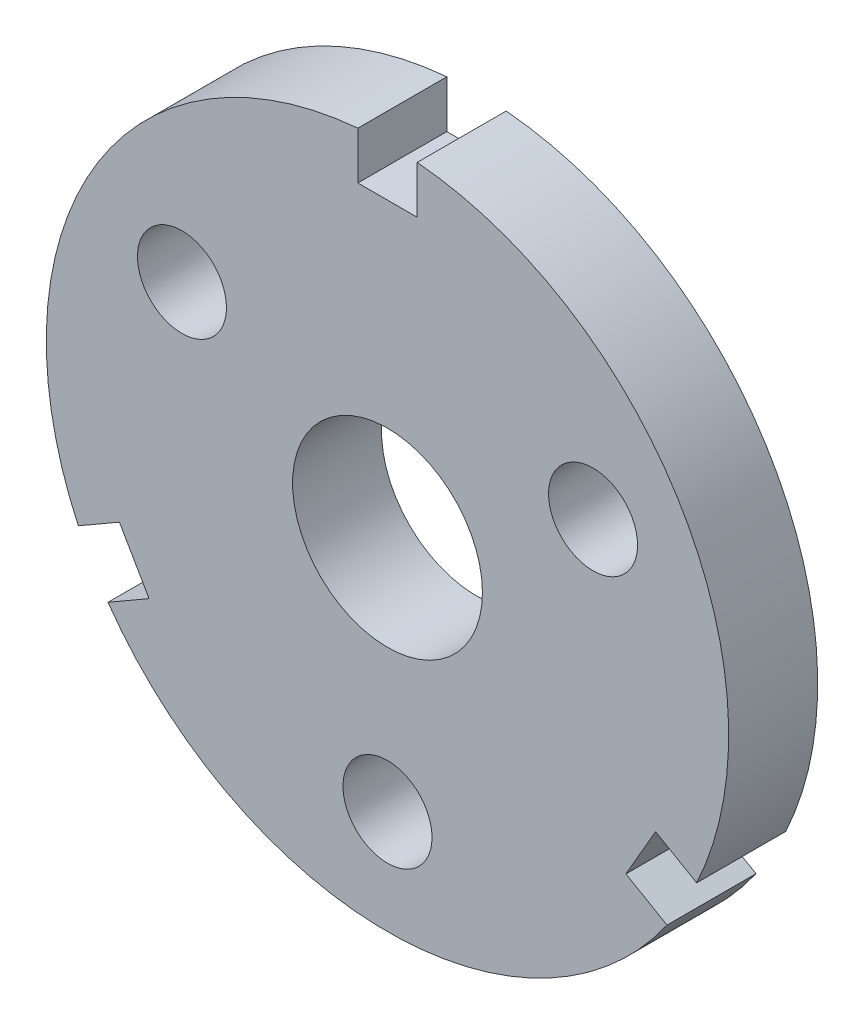
ISO-10303-21;
HEADER;
FILE_DESCRIPTION(('STEP AP214'),'2;1');
FILE_NAME('part.step','',(''),(''),'','','');
FILE_SCHEMA(('AUTOMOTIVE_DESIGN { 1 0 10303 214 1 1 1 1 }'));
ENDSEC;
DATA;
#1=APPLICATION_CONTEXT('core data for automotive mechanical design processes');
#2=APPLICATION_PROTOCOL_DEFINITION('international standard','automotive_design',2000,#1);
#3=PRODUCT_CONTEXT('',#1,'mechanical');
#4=PRODUCT('Part','Part','',(#3));
#5=PRODUCT_RELATED_PRODUCT_CATEGORY('part','',(#4));
#6=PRODUCT_DEFINITION_FORMATION('','',#4);
#7=PRODUCT_DEFINITION_CONTEXT('part definition',#1,'design');
#8=PRODUCT_DEFINITION('design','',#6,#7);
#9=PRODUCT_DEFINITION_SHAPE('','',#8);
#10=(LENGTH_UNIT() NAMED_UNIT(*) SI_UNIT(.MILLI.,.METRE.));
#11=(NAMED_UNIT(*) PLANE_ANGLE_UNIT() SI_UNIT($,.RADIAN.));
#12=(NAMED_UNIT(*) SI_UNIT($,.STERADIAN.) SOLID_ANGLE_UNIT());
#13=UNCERTAINTY_MEASURE_WITH_UNIT(LENGTH_MEASURE(1.E-05),#10,'distance_accuracy_value','');
#14=(GEOMETRIC_REPRESENTATION_CONTEXT(3) GLOBAL_UNCERTAINTY_ASSIGNED_CONTEXT((#13)) GLOBAL_UNIT_ASSIGNED_CONTEXT((#10,
#11,#12)) REPRESENTATION_CONTEXT('',''));
#15=CARTESIAN_POINT('',(0.,0.,0.));
#16=DIRECTION('',(0.,0.,1.));
#17=DIRECTION('',(1.,0.,0.));
#18=AXIS2_PLACEMENT_3D('',#15,#16,#17);
#19=CARTESIAN_POINT('',(0.,0.,15.));
#20=DIRECTION('',(0.,0.,-1.));
#21=DIRECTION('',(-1.,0.,0.));
#22=AXIS2_PLACEMENT_3D('',#19,#20,#21);
#23=CYLINDRICAL_SURFACE('',#22,57.5);
#24=CARTESIAN_POINT('',(0.,0.,0.));
#25=DIRECTION('',(0.,0.,1.));
#26=DIRECTION('',(1.,0.,0.));
#27=AXIS2_PLACEMENT_3D('',#24,#25,#26);
#28=CIRCLE('',#27,57.5);
#29=CARTESIAN_POINT('',(52.1078370824597,-24.3109710745512,0.));
#30=VERTEX_POINT('',#29);
#31=CARTESIAN_POINT('',(4.99999999999981,57.2821961869465,0.));
#32=VERTEX_POINT('',#31);
#33=EDGE_CURVE('E47',#30,#32,#28,.T.);
#34=ORIENTED_EDGE('',*,*,#33,.T.);
#35=DIRECTION('',(0.,0.,1.));
#36=VECTOR('',#35,1.);
#37=CARTESIAN_POINT('',(4.99999999999981,57.2821961869465,0.));
#38=LINE('',#37,#36);
#39=CARTESIAN_POINT('',(4.99999999999981,57.2821961869465,15.));
#40=VERTEX_POINT('',#39);
#41=EDGE_CURVE('E192',#32,#40,#38,.T.);
#42=ORIENTED_EDGE('',*,*,#41,.T.);
#43=CARTESIAN_POINT('',(0.,0.,15.));
#44=DIRECTION('',(0.,0.,1.));
#45=DIRECTION('',(1.,0.,0.));
#46=AXIS2_PLACEMENT_3D('',#43,#44,#45);
#47=CIRCLE('',#46,57.5);
#48=CARTESIAN_POINT('',(52.1078370824597,-24.3109710745512,15.));
#49=VERTEX_POINT('',#48);
#50=EDGE_CURVE('E54',#49,#40,#47,.T.);
#51=ORIENTED_EDGE('',*,*,#50,.F.);
#52=DIRECTION('',(0.,0.,1.));
#53=VECTOR('',#52,1.);
#54=CARTESIAN_POINT('',(52.1078370824597,-24.3109710745512,0.));
#55=LINE('',#54,#53);
#56=EDGE_CURVE('E219',#30,#49,#55,.T.);
#57=ORIENTED_EDGE('',*,*,#56,.F.);
#58=EDGE_LOOP('',(#34,#42,#51,#57));
#59=FACE_BOUND('',#58,.T.);
#60=ADVANCED_FACE('F44',(#59),#23,.T.);
#61=CARTESIAN_POINT('',(-47.1078370824598,-32.9712251123953,0.));
#62=VERTEX_POINT('',#61);
#63=CARTESIAN_POINT('',(47.1078370824599,-32.9712251123953,0.));
#64=VERTEX_POINT('',#63);
#65=EDGE_CURVE('E158',#62,#64,#28,.T.);
#66=ORIENTED_EDGE('',*,*,#65,.T.);
#67=DIRECTION('',(0.,0.,1.));
#68=VECTOR('',#67,1.);
#69=CARTESIAN_POINT('',(47.1078370824599,-32.9712251123953,0.));
#70=LINE('',#69,#68);
#71=CARTESIAN_POINT('',(47.1078370824599,-32.9712251123953,15.));
#72=VERTEX_POINT('',#71);
#73=EDGE_CURVE('E230',#64,#72,#70,.T.);
#74=ORIENTED_EDGE('',*,*,#73,.T.);
#75=CARTESIAN_POINT('',(-47.1078370824598,-32.9712251123953,15.));
#76=VERTEX_POINT('',#75);
#77=EDGE_CURVE('E53',#76,#72,#47,.T.);
#78=ORIENTED_EDGE('',*,*,#77,.F.);
#79=DIRECTION('',(0.,0.,1.));
#80=VECTOR('',#79,1.);
#81=CARTESIAN_POINT('',(-47.1078370824598,-32.9712251123953,0.));
#82=LINE('',#81,#80);
#83=EDGE_CURVE('E201',#62,#76,#82,.T.);
#84=ORIENTED_EDGE('',*,*,#83,.F.);
#85=EDGE_LOOP('',(#66,#74,#78,#84));
#86=FACE_BOUND('',#85,.T.);
#87=ADVANCED_FACE('F273',(#86),#23,.T.);
#88=CARTESIAN_POINT('',(-4.99999999999981,57.2821961869465,15.));
#89=VERTEX_POINT('',#88);
#90=CARTESIAN_POINT('',(-52.1078370824596,-24.3109710745512,15.));
#91=VERTEX_POINT('',#90);
#92=EDGE_CURVE('E11',#89,#91,#47,.T.);
#93=ORIENTED_EDGE('',*,*,#92,.F.);
#94=DIRECTION('',(0.,0.,1.));
#95=VECTOR('',#94,1.);
#96=CARTESIAN_POINT('',(-4.99999999999981,57.2821961869465,0.));
#97=LINE('',#96,#95);
#98=CARTESIAN_POINT('',(-4.99999999999981,57.2821961869465,0.));
#99=VERTEX_POINT('',#98);
#100=EDGE_CURVE('E139',#99,#89,#97,.T.);
#101=ORIENTED_EDGE('',*,*,#100,.F.);
#102=CARTESIAN_POINT('',(-52.1078370824596,-24.3109710745512,0.));
#103=VERTEX_POINT('',#102);
#104=EDGE_CURVE('E147',#99,#103,#28,.T.);
#105=ORIENTED_EDGE('',*,*,#104,.T.);
#106=DIRECTION('',(0.,0.,1.));
#107=VECTOR('',#106,1.);
#108=CARTESIAN_POINT('',(-52.1078370824596,-24.3109710745512,0.));
#109=LINE('',#108,#107);
#110=EDGE_CURVE('E203',#103,#91,#109,.T.);
#111=ORIENTED_EDGE('',*,*,#110,.T.);
#112=EDGE_LOOP('',(#93,#101,#105,#111));
#113=FACE_BOUND('',#112,.T.);
#114=ADVANCED_FACE('F50',(#113),#23,.T.);
#115=CARTESIAN_POINT('',(0.,0.,15.));
#116=DIRECTION('',(0.,0.,1.));
#117=DIRECTION('',(1.,0.,0.));
#118=AXIS2_PLACEMENT_3D('',#115,#116,#117);
#119=PLANE('',#118);
#120=DIRECTION('',(0.,1.,0.));
#121=VECTOR('',#120,1.);
#122=CARTESIAN_POINT('',(4.99999999999981,57.2821961869465,15.));
#123=LINE('',#122,#121);
#124=CARTESIAN_POINT('',(4.99999999999981,49.2821961869465,15.));
#125=VERTEX_POINT('',#124);
#126=EDGE_CURVE('E145',#125,#40,#123,.T.);
#127=ORIENTED_EDGE('',*,*,#126,.F.);
#128=DIRECTION('',(1.,0.,0.));
#129=VECTOR('',#128,1.);
#130=CARTESIAN_POINT('',(-4.99999999999981,49.2821961869465,15.));
#131=LINE('',#130,#129);
#132=CARTESIAN_POINT('',(-4.99999999999981,49.2821961869465,15.));
#133=VERTEX_POINT('',#132);
#134=EDGE_CURVE('E249',#133,#125,#131,.T.);
#135=ORIENTED_EDGE('',*,*,#134,.F.);
#136=DIRECTION('',(0.,-1.,0.));
#137=VECTOR('',#136,1.);
#138=CARTESIAN_POINT('',(-4.99999999999981,49.2821961869465,15.));
#139=LINE('',#138,#137);
#140=EDGE_CURVE('E229',#89,#133,#139,.T.);
#141=ORIENTED_EDGE('',*,*,#140,.F.);
#142=ORIENTED_EDGE('',*,*,#92,.T.);
#143=DIRECTION('',(-0.866025403784438,-0.5,0.));
#144=VECTOR('',#143,1.);
#145=CARTESIAN_POINT('',(-52.1078370824596,-24.3109710745512,15.));
#146=LINE('',#145,#144);
#147=CARTESIAN_POINT('',(-45.1796338521841,-20.3109710745512,15.));
#148=VERTEX_POINT('',#147);
#149=EDGE_CURVE('E206',#148,#91,#146,.T.);
#150=ORIENTED_EDGE('',*,*,#149,.F.);
#151=DIRECTION('',(-0.500000000000001,0.866025403784438,0.));
#152=VECTOR('',#151,1.);
#153=CARTESIAN_POINT('',(-40.1796338521843,-28.9712251123953,15.));
#154=LINE('',#153,#152);
#155=CARTESIAN_POINT('',(-40.1796338521843,-28.9712251123953,15.));
#156=VERTEX_POINT('',#155);
#157=EDGE_CURVE('E207',#156,#148,#154,.T.);
#158=ORIENTED_EDGE('',*,*,#157,.F.);
#159=DIRECTION('',(0.866025403784438,0.5,0.));
#160=VECTOR('',#159,1.);
#161=CARTESIAN_POINT('',(-40.1796338521843,-28.9712251123953,15.));
#162=LINE('',#161,#160);
#163=EDGE_CURVE('E215',#76,#156,#162,.T.);
#164=ORIENTED_EDGE('',*,*,#163,.F.);
#165=ORIENTED_EDGE('',*,*,#77,.T.);
#166=DIRECTION('',(0.866025403784439,-0.499999999999999,0.));
#167=VECTOR('',#166,1.);
#168=CARTESIAN_POINT('',(47.1078370824599,-32.9712251123953,15.));
#169=LINE('',#168,#167);
#170=CARTESIAN_POINT('',(40.1796338521843,-28.9712251123953,15.));
#171=VERTEX_POINT('',#170);
#172=EDGE_CURVE('E233',#171,#72,#169,.T.);
#173=ORIENTED_EDGE('',*,*,#172,.F.);
#174=DIRECTION('',(-0.5,-0.866025403784439,0.));
#175=VECTOR('',#174,1.);
#176=CARTESIAN_POINT('',(45.1796338521842,-20.3109710745512,15.));
#177=LINE('',#176,#175);
#178=CARTESIAN_POINT('',(45.1796338521842,-20.3109710745512,15.));
#179=VERTEX_POINT('',#178);
#180=EDGE_CURVE('E234',#179,#171,#177,.T.);
#181=ORIENTED_EDGE('',*,*,#180,.F.);
#182=DIRECTION('',(-0.866025403784439,0.5,0.));
#183=VECTOR('',#182,1.);
#184=CARTESIAN_POINT('',(45.1796338521842,-20.3109710745512,15.));
#185=LINE('',#184,#183);
#186=EDGE_CURVE('E202',#49,#179,#185,.T.);
#187=ORIENTED_EDGE('',*,*,#186,.F.);
#188=ORIENTED_EDGE('',*,*,#50,.T.);
#189=EDGE_LOOP('',(#127,#135,#141,#142,#150,#158,#164,#165,#173,#181,#187,#188));
#190=FACE_BOUND('',#189,.T.);
#191=CARTESIAN_POINT('',(0.,0.,15.));
#192=DIRECTION('',(0.,0.,1.));
#193=DIRECTION('',(1.,0.,0.));
#194=AXIS2_PLACEMENT_3D('',#191,#192,#193);
#195=CIRCLE('',#194,16.);
#196=CARTESIAN_POINT('',(16.,0.,15.));
#197=VERTEX_POINT('',#196);
#198=EDGE_CURVE('E178',#197,#197,#195,.T.);
#199=ORIENTED_EDGE('',*,*,#198,.F.);
#200=EDGE_LOOP('',(#199));
#201=FACE_BOUND('',#200,.T.);
#202=CARTESIAN_POINT('',(-34.6410161513775,20.,15.));
#203=DIRECTION('',(0.,0.,1.));
#204=DIRECTION('',(1.,0.,0.));
#205=AXIS2_PLACEMENT_3D('',#202,#203,#204);
#206=CIRCLE('',#205,7.5);
#207=CARTESIAN_POINT('',(-27.1410161513775,20.,15.));
#208=VERTEX_POINT('',#207);
#209=EDGE_CURVE('E169',#208,#208,#206,.T.);
#210=ORIENTED_EDGE('',*,*,#209,.F.);
#211=EDGE_LOOP('',(#210));
#212=FACE_BOUND('',#211,.T.);
#213=CARTESIAN_POINT('',(0.,-40.,15.));
#214=DIRECTION('',(0.,0.,1.));
#215=DIRECTION('',(1.,0.,0.));
#216=AXIS2_PLACEMENT_3D('',#213,#214,#215);
#217=CIRCLE('',#216,7.5);
#218=CARTESIAN_POINT('',(7.5,-40.,15.));
#219=VERTEX_POINT('',#218);
#220=EDGE_CURVE('E182',#219,#219,#217,.T.);
#221=ORIENTED_EDGE('',*,*,#220,.F.);
#222=EDGE_LOOP('',(#221));
#223=FACE_BOUND('',#222,.T.);
#224=CARTESIAN_POINT('',(34.6410161513775,20.0000000000001,15.));
#225=DIRECTION('',(0.,0.,1.));
#226=DIRECTION('',(1.,0.,0.));
#227=AXIS2_PLACEMENT_3D('',#224,#225,#226);
#228=CIRCLE('',#227,7.49999999999999);
#229=CARTESIAN_POINT('',(42.1410161513775,20.0000000000001,15.));
#230=VERTEX_POINT('',#229);
#231=EDGE_CURVE('E190',#230,#230,#228,.T.);
#232=ORIENTED_EDGE('',*,*,#231,.F.);
#233=EDGE_LOOP('',(#232));
#234=FACE_BOUND('',#233,.T.);
#235=ADVANCED_FACE('F265',(#190,#201,#212,#223,#234),#119,.T.);
#236=CARTESIAN_POINT('',(0.,0.,0.));
#237=DIRECTION('',(0.,0.,1.));
#238=DIRECTION('',(1.,0.,0.));
#239=AXIS2_PLACEMENT_3D('',#236,#237,#238);
#240=PLANE('',#239);
#241=DIRECTION('',(1.,0.,0.));
#242=VECTOR('',#241,1.);
#243=CARTESIAN_POINT('',(-4.99999999999981,49.2821961869465,0.));
#244=LINE('',#243,#242);
#245=CARTESIAN_POINT('',(-4.99999999999981,49.2821961869465,0.));
#246=VERTEX_POINT('',#245);
#247=CARTESIAN_POINT('',(4.99999999999981,49.2821961869465,0.));
#248=VERTEX_POINT('',#247);
#249=EDGE_CURVE('E65',#246,#248,#244,.T.);
#250=ORIENTED_EDGE('',*,*,#249,.T.);
#251=DIRECTION('',(0.,1.,0.));
#252=VECTOR('',#251,1.);
#253=CARTESIAN_POINT('',(4.99999999999981,57.2821961869465,0.));
#254=LINE('',#253,#252);
#255=EDGE_CURVE('E151',#248,#32,#254,.T.);
#256=ORIENTED_EDGE('',*,*,#255,.T.);
#257=ORIENTED_EDGE('',*,*,#33,.F.);
#258=DIRECTION('',(-0.866025403784439,0.5,0.));
#259=VECTOR('',#258,1.);
#260=CARTESIAN_POINT('',(45.1796338521842,-20.3109710745512,0.));
#261=LINE('',#260,#259);
#262=CARTESIAN_POINT('',(45.1796338521842,-20.3109710745512,0.));
#263=VERTEX_POINT('',#262);
#264=EDGE_CURVE('E231',#30,#263,#261,.T.);
#265=ORIENTED_EDGE('',*,*,#264,.T.);
#266=DIRECTION('',(-0.5,-0.866025403784439,0.));
#267=VECTOR('',#266,1.);
#268=CARTESIAN_POINT('',(45.1796338521842,-20.3109710745512,0.));
#269=LINE('',#268,#267);
#270=CARTESIAN_POINT('',(40.1796338521843,-28.9712251123953,0.));
#271=VERTEX_POINT('',#270);
#272=EDGE_CURVE('E67',#263,#271,#269,.T.);
#273=ORIENTED_EDGE('',*,*,#272,.T.);
#274=DIRECTION('',(0.866025403784439,-0.499999999999999,0.));
#275=VECTOR('',#274,1.);
#276=CARTESIAN_POINT('',(47.1078370824599,-32.9712251123953,0.));
#277=LINE('',#276,#275);
#278=EDGE_CURVE('E224',#271,#64,#277,.T.);
#279=ORIENTED_EDGE('',*,*,#278,.T.);
#280=ORIENTED_EDGE('',*,*,#65,.F.);
#281=DIRECTION('',(0.866025403784438,0.5,0.));
#282=VECTOR('',#281,1.);
#283=CARTESIAN_POINT('',(-40.1796338521843,-28.9712251123953,0.));
#284=LINE('',#283,#282);
#285=CARTESIAN_POINT('',(-40.1796338521843,-28.9712251123953,0.));
#286=VERTEX_POINT('',#285);
#287=EDGE_CURVE('E208',#62,#286,#284,.T.);
#288=ORIENTED_EDGE('',*,*,#287,.T.);
#289=DIRECTION('',(-0.500000000000001,0.866025403784438,0.));
#290=VECTOR('',#289,1.);
#291=CARTESIAN_POINT('',(-40.1796338521843,-28.9712251123953,0.));
#292=LINE('',#291,#290);
#293=CARTESIAN_POINT('',(-45.1796338521841,-20.3109710745512,0.));
#294=VERTEX_POINT('',#293);
#295=EDGE_CURVE('E216',#286,#294,#292,.T.);
#296=ORIENTED_EDGE('',*,*,#295,.T.);
#297=DIRECTION('',(-0.866025403784438,-0.5,0.));
#298=VECTOR('',#297,1.);
#299=CARTESIAN_POINT('',(-52.1078370824596,-24.3109710745512,0.));
#300=LINE('',#299,#298);
#301=EDGE_CURVE('E160',#294,#103,#300,.T.);
#302=ORIENTED_EDGE('',*,*,#301,.T.);
#303=ORIENTED_EDGE('',*,*,#104,.F.);
#304=DIRECTION('',(0.,-1.,0.));
#305=VECTOR('',#304,1.);
#306=CARTESIAN_POINT('',(-4.99999999999981,49.2821961869465,0.));
#307=LINE('',#306,#305);
#308=EDGE_CURVE('E134',#99,#246,#307,.T.);
#309=ORIENTED_EDGE('',*,*,#308,.T.);
#310=EDGE_LOOP('',(#250,#256,#257,#265,#273,#279,#280,#288,#296,#302,#303,#309));
#311=FACE_BOUND('',#310,.T.);
#312=CARTESIAN_POINT('',(0.,0.,0.));
#313=DIRECTION('',(0.,0.,1.));
#314=DIRECTION('',(1.,0.,0.));
#315=AXIS2_PLACEMENT_3D('',#312,#313,#314);
#316=CIRCLE('',#315,16.);
#317=CARTESIAN_POINT('',(16.,0.,0.));
#318=VERTEX_POINT('',#317);
#319=EDGE_CURVE('E188',#318,#318,#316,.T.);
#320=ORIENTED_EDGE('',*,*,#319,.T.);
#321=EDGE_LOOP('',(#320));
#322=FACE_BOUND('',#321,.T.);
#323=CARTESIAN_POINT('',(-34.6410161513775,20.,0.));
#324=DIRECTION('',(0.,0.,1.));
#325=DIRECTION('',(1.,0.,0.));
#326=AXIS2_PLACEMENT_3D('',#323,#324,#325);
#327=CIRCLE('',#326,7.5);
#328=CARTESIAN_POINT('',(-27.1410161513775,20.,0.));
#329=VERTEX_POINT('',#328);
#330=EDGE_CURVE('E165',#329,#329,#327,.T.);
#331=ORIENTED_EDGE('',*,*,#330,.T.);
#332=EDGE_LOOP('',(#331));
#333=FACE_BOUND('',#332,.T.);
#334=CARTESIAN_POINT('',(0.,-40.,0.));
#335=DIRECTION('',(0.,0.,1.));
#336=DIRECTION('',(1.,0.,0.));
#337=AXIS2_PLACEMENT_3D('',#334,#335,#336);
#338=CIRCLE('',#337,7.5);
#339=CARTESIAN_POINT('',(7.5,-40.,0.));
#340=VERTEX_POINT('',#339);
#341=EDGE_CURVE('E172',#340,#340,#338,.T.);
#342=ORIENTED_EDGE('',*,*,#341,.T.);
#343=EDGE_LOOP('',(#342));
#344=FACE_BOUND('',#343,.T.);
#345=CARTESIAN_POINT('',(34.6410161513775,20.0000000000001,0.));
#346=DIRECTION('',(0.,0.,1.));
#347=DIRECTION('',(1.,0.,0.));
#348=AXIS2_PLACEMENT_3D('',#345,#346,#347);
#349=CIRCLE('',#348,7.49999999999999);
#350=CARTESIAN_POINT('',(42.1410161513775,20.0000000000001,0.));
#351=VERTEX_POINT('',#350);
#352=EDGE_CURVE('E184',#351,#351,#349,.T.);
#353=ORIENTED_EDGE('',*,*,#352,.T.);
#354=EDGE_LOOP('',(#353));
#355=FACE_BOUND('',#354,.T.);
#356=ADVANCED_FACE('F152',(#311,#322,#333,#344,#355),#240,.F.);
#357=CARTESIAN_POINT('',(34.6410161513775,20.0000000000001,0.));
#358=DIRECTION('',(0.,0.,1.));
#359=DIRECTION('',(1.,0.,0.));
#360=AXIS2_PLACEMENT_3D('',#357,#358,#359);
#361=CYLINDRICAL_SURFACE('',#360,7.49999999999999);
#362=ORIENTED_EDGE('',*,*,#352,.F.);
#363=EDGE_LOOP('',(#362));
#364=FACE_BOUND('',#363,.T.);
#365=ORIENTED_EDGE('',*,*,#231,.T.);
#366=EDGE_LOOP('',(#365));
#367=FACE_BOUND('',#366,.T.);
#368=ADVANCED_FACE('F309',(#364,#367),#361,.F.);
#369=CARTESIAN_POINT('',(0.,-40.,0.));
#370=DIRECTION('',(0.,0.,1.));
#371=DIRECTION('',(1.,0.,0.));
#372=AXIS2_PLACEMENT_3D('',#369,#370,#371);
#373=CYLINDRICAL_SURFACE('',#372,7.5);
#374=ORIENTED_EDGE('',*,*,#341,.F.);
#375=EDGE_LOOP('',(#374));
#376=FACE_BOUND('',#375,.T.);
#377=ORIENTED_EDGE('',*,*,#220,.T.);
#378=EDGE_LOOP('',(#377));
#379=FACE_BOUND('',#378,.T.);
#380=ADVANCED_FACE('F314',(#376,#379),#373,.F.);
#381=CARTESIAN_POINT('',(-34.6410161513775,20.,0.));
#382=DIRECTION('',(0.,0.,1.));
#383=DIRECTION('',(1.,0.,0.));
#384=AXIS2_PLACEMENT_3D('',#381,#382,#383);
#385=CYLINDRICAL_SURFACE('',#384,7.5);
#386=ORIENTED_EDGE('',*,*,#330,.F.);
#387=EDGE_LOOP('',(#386));
#388=FACE_BOUND('',#387,.T.);
#389=ORIENTED_EDGE('',*,*,#209,.T.);
#390=EDGE_LOOP('',(#389));
#391=FACE_BOUND('',#390,.T.);
#392=ADVANCED_FACE('F318',(#388,#391),#385,.F.);
#393=CARTESIAN_POINT('',(0.,0.,0.));
#394=DIRECTION('',(0.,0.,1.));
#395=DIRECTION('',(1.,0.,0.));
#396=AXIS2_PLACEMENT_3D('',#393,#394,#395);
#397=CYLINDRICAL_SURFACE('',#396,16.);
#398=ORIENTED_EDGE('',*,*,#319,.F.);
#399=EDGE_LOOP('',(#398));
#400=FACE_BOUND('',#399,.T.);
#401=ORIENTED_EDGE('',*,*,#198,.T.);
#402=EDGE_LOOP('',(#401));
#403=FACE_BOUND('',#402,.T.);
#404=ADVANCED_FACE('F325',(#400,#403),#397,.F.);
#405=CARTESIAN_POINT('',(-40.1796338521843,-28.9712251123953,0.));
#406=DIRECTION('',(0.5,-0.866025403784438,0.));
#407=DIRECTION('',(0.866025403784439,0.5,0.));
#408=AXIS2_PLACEMENT_3D('',#405,#406,#407);
#409=PLANE('',#408);
#410=ORIENTED_EDGE('',*,*,#163,.T.);
#411=DIRECTION('',(0.,0.,1.));
#412=VECTOR('',#411,1.);
#413=CARTESIAN_POINT('',(-40.1796338521843,-28.9712251123953,0.));
#414=LINE('',#413,#412);
#415=EDGE_CURVE('E197',#286,#156,#414,.T.);
#416=ORIENTED_EDGE('',*,*,#415,.F.);
#417=ORIENTED_EDGE('',*,*,#287,.F.);
#418=ORIENTED_EDGE('',*,*,#83,.T.);
#419=EDGE_LOOP('',(#410,#416,#417,#418));
#420=FACE_BOUND('',#419,.T.);
#421=ADVANCED_FACE('F276',(#420),#409,.F.);
#422=CARTESIAN_POINT('',(-52.1078370824596,-24.3109710745512,0.));
#423=DIRECTION('',(-0.5,0.866025403784438,0.));
#424=DIRECTION('',(-0.866025403784438,-0.5,0.));
#425=AXIS2_PLACEMENT_3D('',#422,#423,#424);
#426=PLANE('',#425);
#427=ORIENTED_EDGE('',*,*,#149,.T.);
#428=ORIENTED_EDGE('',*,*,#110,.F.);
#429=ORIENTED_EDGE('',*,*,#301,.F.);
#430=DIRECTION('',(0.,0.,1.));
#431=VECTOR('',#430,1.);
#432=CARTESIAN_POINT('',(-45.1796338521841,-20.3109710745512,0.));
#433=LINE('',#432,#431);
#434=EDGE_CURVE('E200',#294,#148,#433,.T.);
#435=ORIENTED_EDGE('',*,*,#434,.T.);
#436=EDGE_LOOP('',(#427,#428,#429,#435));
#437=FACE_BOUND('',#436,.T.);
#438=ADVANCED_FACE('F290',(#437),#426,.F.);
#439=CARTESIAN_POINT('',(-40.1796338521843,-28.9712251123953,0.));
#440=DIRECTION('',(0.866025403784438,0.500000000000001,0.));
#441=DIRECTION('',(-0.500000000000001,0.866025403784438,0.));
#442=AXIS2_PLACEMENT_3D('',#439,#440,#441);
#443=PLANE('',#442);
#444=ORIENTED_EDGE('',*,*,#157,.T.);
#445=ORIENTED_EDGE('',*,*,#434,.F.);
#446=ORIENTED_EDGE('',*,*,#295,.F.);
#447=ORIENTED_EDGE('',*,*,#415,.T.);
#448=EDGE_LOOP('',(#444,#445,#446,#447));
#449=FACE_BOUND('',#448,.T.);
#450=ADVANCED_FACE('F283',(#449),#443,.F.);
#451=CARTESIAN_POINT('',(47.1078370824599,-32.9712251123953,0.));
#452=DIRECTION('',(-0.499999999999999,-0.866025403784439,0.));
#453=DIRECTION('',(0.86602540378444,-0.499999999999999,0.));
#454=AXIS2_PLACEMENT_3D('',#451,#452,#453);
#455=PLANE('',#454);
#456=ORIENTED_EDGE('',*,*,#172,.T.);
#457=ORIENTED_EDGE('',*,*,#73,.F.);
#458=ORIENTED_EDGE('',*,*,#278,.F.);
#459=DIRECTION('',(0.,0.,1.));
#460=VECTOR('',#459,1.);
#461=CARTESIAN_POINT('',(40.1796338521843,-28.9712251123953,0.));
#462=LINE('',#461,#460);
#463=EDGE_CURVE('E223',#271,#171,#462,.T.);
#464=ORIENTED_EDGE('',*,*,#463,.T.);
#465=EDGE_LOOP('',(#456,#457,#458,#464));
#466=FACE_BOUND('',#465,.T.);
#467=ADVANCED_FACE('F332',(#466),#455,.F.);
#468=CARTESIAN_POINT('',(45.1796338521842,-20.3109710745512,0.));
#469=DIRECTION('',(-0.866025403784439,0.5,0.));
#470=DIRECTION('',(-0.5,-0.866025403784439,0.));
#471=AXIS2_PLACEMENT_3D('',#468,#469,#470);
#472=PLANE('',#471);
#473=ORIENTED_EDGE('',*,*,#180,.T.);
#474=ORIENTED_EDGE('',*,*,#463,.F.);
#475=ORIENTED_EDGE('',*,*,#272,.F.);
#476=DIRECTION('',(0.,0.,1.));
#477=VECTOR('',#476,1.);
#478=CARTESIAN_POINT('',(45.1796338521842,-20.3109710745512,0.));
#479=LINE('',#478,#477);
#480=EDGE_CURVE('E225',#263,#179,#479,.T.);
#481=ORIENTED_EDGE('',*,*,#480,.T.);
#482=EDGE_LOOP('',(#473,#474,#475,#481));
#483=FACE_BOUND('',#482,.T.);
#484=ADVANCED_FACE('F336',(#483),#472,.F.);
#485=CARTESIAN_POINT('',(45.1796338521842,-20.3109710745512,0.));
#486=DIRECTION('',(0.5,0.866025403784439,0.));
#487=DIRECTION('',(-0.866025403784439,0.5,0.));
#488=AXIS2_PLACEMENT_3D('',#485,#486,#487);
#489=PLANE('',#488);
#490=ORIENTED_EDGE('',*,*,#186,.T.);
#491=ORIENTED_EDGE('',*,*,#480,.F.);
#492=ORIENTED_EDGE('',*,*,#264,.F.);
#493=ORIENTED_EDGE('',*,*,#56,.T.);
#494=EDGE_LOOP('',(#490,#491,#492,#493));
#495=FACE_BOUND('',#494,.T.);
#496=ADVANCED_FACE('F268',(#495),#489,.F.);
#497=CARTESIAN_POINT('',(4.99999999999981,57.2821961869465,0.));
#498=DIRECTION('',(1.,0.,0.));
#499=DIRECTION('',(0.,1.,0.));
#500=AXIS2_PLACEMENT_3D('',#497,#498,#499);
#501=PLANE('',#500);
#502=ORIENTED_EDGE('',*,*,#126,.T.);
#503=ORIENTED_EDGE('',*,*,#41,.F.);
#504=ORIENTED_EDGE('',*,*,#255,.F.);
#505=DIRECTION('',(0.,0.,1.));
#506=VECTOR('',#505,1.);
#507=CARTESIAN_POINT('',(4.99999999999981,49.2821961869465,0.));
#508=LINE('',#507,#506);
#509=EDGE_CURVE('E244',#248,#125,#508,.T.);
#510=ORIENTED_EDGE('',*,*,#509,.T.);
#511=EDGE_LOOP('',(#502,#503,#504,#510));
#512=FACE_BOUND('',#511,.T.);
#513=ADVANCED_FACE('F260',(#512),#501,.F.);
#514=CARTESIAN_POINT('',(-4.99999999999981,49.2821961869465,0.));
#515=DIRECTION('',(0.,-1.,0.));
#516=DIRECTION('',(0.,0.,-1.));
#517=AXIS2_PLACEMENT_3D('',#514,#515,#516);
#518=PLANE('',#517);
#519=ORIENTED_EDGE('',*,*,#134,.T.);
#520=ORIENTED_EDGE('',*,*,#509,.F.);
#521=ORIENTED_EDGE('',*,*,#249,.F.);
#522=DIRECTION('',(0.,0.,1.));
#523=VECTOR('',#522,1.);
#524=CARTESIAN_POINT('',(-4.99999999999981,49.2821961869465,0.));
#525=LINE('',#524,#523);
#526=EDGE_CURVE('E143',#246,#133,#525,.T.);
#527=ORIENTED_EDGE('',*,*,#526,.T.);
#528=EDGE_LOOP('',(#519,#520,#521,#527));
#529=FACE_BOUND('',#528,.T.);
#530=ADVANCED_FACE('F286',(#529),#518,.F.);
#531=CARTESIAN_POINT('',(-4.99999999999981,49.2821961869465,0.));
#532=DIRECTION('',(-1.,0.,0.));
#533=DIRECTION('',(0.,0.,1.));
#534=AXIS2_PLACEMENT_3D('',#531,#532,#533);
#535=PLANE('',#534);
#536=ORIENTED_EDGE('',*,*,#140,.T.);
#537=ORIENTED_EDGE('',*,*,#526,.F.);
#538=ORIENTED_EDGE('',*,*,#308,.F.);
#539=ORIENTED_EDGE('',*,*,#100,.T.);
#540=EDGE_LOOP('',(#536,#537,#538,#539));
#541=FACE_BOUND('',#540,.T.);
#542=ADVANCED_FACE('F136',(#541),#535,.F.);
#543=CLOSED_SHELL('',(#60,#87,#114,#235,#356,#368,#380,#392,#404,#421,#438,#450,#467,#484,#496,
#513,#530,#542));
#544=MANIFOLD_SOLID_BREP('B2',#543);
#545=ADVANCED_BREP_SHAPE_REPRESENTATION('',(#18,#544),#14);
#546=SHAPE_DEFINITION_REPRESENTATION(#9,#545);
ENDSEC;
END-ISO-10303-21;
